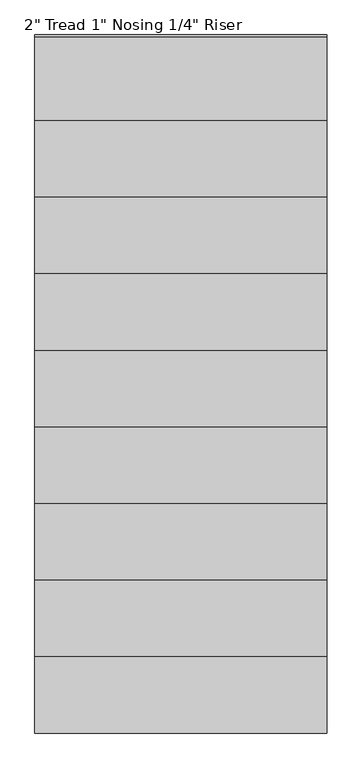
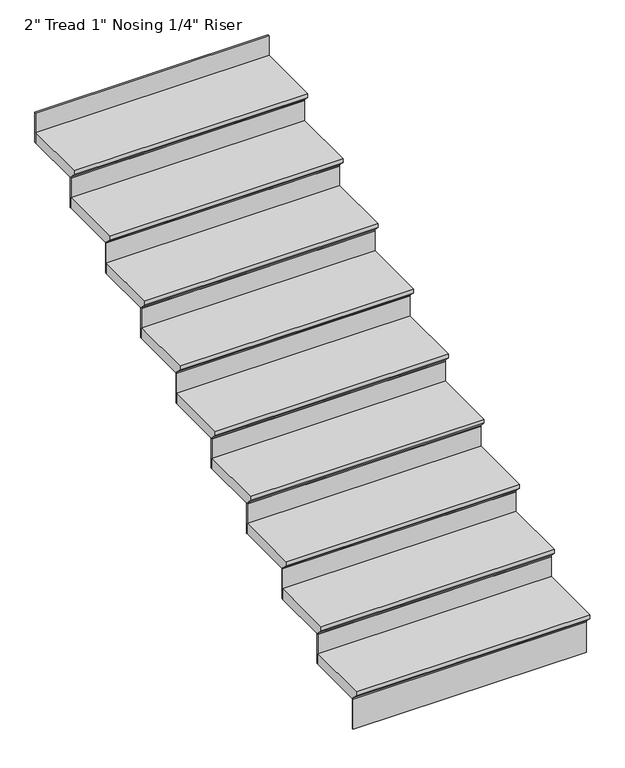
"""IFC4 building model written with IfcOpenShell, lengths in millimetres: stair flight geometry."""

from ifc_helpers import new_model, si_unit, frame, origin, place, context, project, spatial, polyline, outline, extrude, source, transform, mapped, element, save


def stair_flight_4fea8275(model_context):
    return source(origin(), model_context, "Body", "SweptSolid", [
        extrude(outline(polyline([(9995.9922903, 4800.6), (10300.7922903, 4800.6), (10300.7922903, 4749.8), (10021.3922903, 4749.8), (10021.3922903, 4756.15), (9995.9922903, 4781.55), (9995.9922903, 4800.6)])), frame((-17359.2847893, 0.0, 0.0), z_axis=(1.0, 0.0, 0.0), x_axis=(0.0, 1.0, 0.0)), (0.0, 0.0, 1.0), 1066.8),
        extrude(outline(polyline([(-16292.4847893, 10027.7422903), (-16292.4847893, 10021.3922903), (-17359.2847893, 10021.3922903), (-17359.2847893, 10027.7422903), (-16292.4847893, 10027.7422903)])), frame((0.0, 0.0, 4604.3272727), z_axis=(0.0, 0.0, 1.0), x_axis=(1.0, 0.0, 0.0)), (0.0, 0.0, 1.0), 145.4727273),
        extrude(outline(polyline([(-16292.4847893, 10307.1422903), (-16292.4847893, 10300.7922903), (-17359.2847893, 10300.7922903), (-17359.2847893, 10307.1422903), (-16292.4847893, 10307.1422903)])), frame((0.0, 0.0, 4749.8), z_axis=(0.0, 0.0, 1.0), x_axis=(1.0, 0.0, 0.0)), (0.0, 0.0, 1.0), 145.4727273),
        extrude(outline(polyline([(10275.3922903, 4946.0727273), (10580.1922903, 4946.0727273), (10580.1922903, 4895.2727273), (10300.7922903, 4895.2727273), (10300.7922903, 4901.6227273), (10275.3922903, 4927.0227273), (10275.3922903, 4946.0727273)])), frame((-17359.2847893, 0.0, 0.0), z_axis=(1.0, 0.0, 0.0), x_axis=(0.0, 1.0, 0.0)), (0.0, 0.0, 1.0), 1066.8),
        extrude(outline(polyline([(-16292.4847893, 10586.5422903), (-16292.4847893, 10580.1922903), (-17359.2847893, 10580.1922903), (-17359.2847893, 10586.5422903), (-16292.4847893, 10586.5422903)])), frame((0.0, 0.0, 4895.2727273), z_axis=(0.0, 0.0, 1.0), x_axis=(1.0, 0.0, 0.0)), (0.0, 0.0, 1.0), 145.4727273),
        extrude(outline(polyline([(10554.7922903, 5091.5454545), (10859.5922903, 5091.5454545), (10859.5922903, 5040.7454545), (10580.1922903, 5040.7454545), (10580.1922903, 5047.0954545), (10554.7922903, 5072.4954545), (10554.7922903, 5091.5454545)])), frame((-17359.2847893, 0.0, 0.0), z_axis=(1.0, 0.0, 0.0), x_axis=(0.0, 1.0, 0.0)), (0.0, 0.0, 1.0), 1066.8),
        extrude(outline(polyline([(-16292.4847893, 10865.9422903), (-16292.4847893, 10859.5922903), (-17359.2847893, 10859.5922903), (-17359.2847893, 10865.9422903), (-16292.4847893, 10865.9422903)])), frame((0.0, 0.0, 5040.7454545), z_axis=(0.0, 0.0, 1.0), x_axis=(1.0, 0.0, 0.0)), (0.0, 0.0, 1.0), 145.4727273),
        extrude(outline(polyline([(10834.1922903, 5237.0181818), (11138.9922903, 5237.0181818), (11138.9922903, 5186.2181818), (10859.5922903, 5186.2181818), (10859.5922903, 5192.5681818), (10834.1922903, 5217.9681818), (10834.1922903, 5237.0181818)])), frame((-17359.2847893, 0.0, 0.0), z_axis=(1.0, 0.0, 0.0), x_axis=(0.0, 1.0, 0.0)), (0.0, 0.0, 1.0), 1066.8),
        extrude(outline(polyline([(-16292.4847893, 11145.3422903), (-16292.4847893, 11138.9922903), (-17359.2847893, 11138.9922903), (-17359.2847893, 11145.3422903), (-16292.4847893, 11145.3422903)])), frame((0.0, 0.0, 5186.2181818), z_axis=(0.0, 0.0, 1.0), x_axis=(1.0, 0.0, 0.0)), (0.0, 0.0, 1.0), 145.4727273),
        extrude(outline(polyline([(11113.5922903, 5382.4909091), (11418.3922903, 5382.4909091), (11418.3922903, 5331.6909091), (11138.9922903, 5331.6909091), (11138.9922903, 5338.0409091), (11113.5922903, 5363.4409091), (11113.5922903, 5382.4909091)])), frame((-17359.2847893, 0.0, 0.0), z_axis=(1.0, 0.0, 0.0), x_axis=(0.0, 1.0, 0.0)), (0.0, 0.0, 1.0), 1066.8),
        extrude(outline(polyline([(-16292.4847893, 11424.7422903), (-16292.4847893, 11418.3922903), (-17359.2847893, 11418.3922903), (-17359.2847893, 11424.7422903), (-16292.4847893, 11424.7422903)])), frame((0.0, 0.0, 5331.6909091), z_axis=(0.0, 0.0, 1.0), x_axis=(1.0, 0.0, 0.0)), (0.0, 0.0, 1.0), 145.4727273),
        extrude(outline(polyline([(11392.9922903, 5527.9636364), (11697.7922903, 5527.9636364), (11697.7922903, 5477.1636364), (11418.3922903, 5477.1636364), (11418.3922903, 5483.5136364), (11392.9922903, 5508.9136364), (11392.9922903, 5527.9636364)])), frame((-17359.2847893, 0.0, 0.0), z_axis=(1.0, 0.0, 0.0), x_axis=(0.0, 1.0, 0.0)), (0.0, 0.0, 1.0), 1066.8),
        extrude(outline(polyline([(-16292.4847893, 11704.1422903), (-16292.4847893, 11697.7922903), (-17359.2847893, 11697.7922903), (-17359.2847893, 11704.1422903), (-16292.4847893, 11704.1422903)])), frame((0.0, 0.0, 5477.1636364), z_axis=(0.0, 0.0, 1.0), x_axis=(1.0, 0.0, 0.0)), (0.0, 0.0, 1.0), 145.4727273),
        extrude(outline(polyline([(11672.3922903, 5673.4363636), (11977.1922903, 5673.4363636), (11977.1922903, 5622.6363636), (11697.7922903, 5622.6363636), (11697.7922903, 5628.9863636), (11672.3922903, 5654.3863636), (11672.3922903, 5673.4363636)])), frame((-17359.2847893, 0.0, 0.0), z_axis=(1.0, 0.0, 0.0), x_axis=(0.0, 1.0, 0.0)), (0.0, 0.0, 1.0), 1066.8),
        extrude(outline(polyline([(-16292.4847893, 11983.5422903), (-16292.4847893, 11977.1922903), (-17359.2847893, 11977.1922903), (-17359.2847893, 11983.5422903), (-16292.4847893, 11983.5422903)])), frame((0.0, 0.0, 5622.6363636), z_axis=(0.0, 0.0, 1.0), x_axis=(1.0, 0.0, 0.0)), (0.0, 0.0, 1.0), 145.4727273),
        extrude(outline(polyline([(11951.7922903, 5818.9090909), (12256.5922903, 5818.9090909), (12256.5922903, 5768.1090909), (11977.1922903, 5768.1090909), (11977.1922903, 5774.4590909), (11951.7922903, 5799.8590909), (11951.7922903, 5818.9090909)])), frame((-17359.2847893, 0.0, 0.0), z_axis=(1.0, 0.0, 0.0), x_axis=(0.0, 1.0, 0.0)), (0.0, 0.0, 1.0), 1066.8),
        extrude(outline(polyline([(-16292.4847893, 12262.9422903), (-16292.4847893, 12256.5922903), (-17359.2847893, 12256.5922903), (-17359.2847893, 12262.9422903), (-16292.4847893, 12262.9422903)])), frame((0.0, 0.0, 5768.1090909), z_axis=(0.0, 0.0, 1.0), x_axis=(1.0, 0.0, 0.0)), (0.0, 0.0, 1.0), 145.4727273),
        extrude(outline(polyline([(-16292.4847893, 12542.3422903), (-16292.4847893, 12535.9922903), (-17359.2847893, 12535.9922903), (-17359.2847893, 12542.3422903), (-16292.4847893, 12542.3422903)])), frame((0.0, 0.0, 5913.5818182), z_axis=(0.0, 0.0, 1.0), x_axis=(1.0, 0.0, 0.0)), (0.0, 0.0, 1.0), 145.4727273),
        extrude(outline(polyline([(12231.1922903, 5964.3818182), (12535.9922903, 5964.3818182), (12535.9922903, 5913.5818182), (12256.5922903, 5913.5818182), (12256.5922903, 5919.9318182), (12231.1922903, 5945.3318182), (12231.1922903, 5964.3818182)])), frame((-17359.2847893, 0.0, 0.0), z_axis=(1.0, 0.0, 0.0), x_axis=(0.0, 1.0, 0.0)), (0.0, 0.0, 1.0), 1066.8),
    ])


if __name__ == "__main__":
    model = new_model("IFC4")
    model_context = context("Model", 3, world=origin())
    ifc_project = project(units=[si_unit("LENGTHUNIT", "METRE", prefix="MILLI")], contexts=[model_context])
    site = spatial("IfcSite", under=ifc_project)
    building = spatial("IfcBuilding", under=site)
    placement = place(None, origin())
    stair_flight_shape = stair_flight_4fea8275(model_context)
    element("IfcStairFlight", 1, ObjectType="2\" Tread 1\" Nosing 1/4\" Riser", at=placement, inside=building, context=model_context, shape_type="MappedRepresentation", body=[
        mapped(stair_flight_shape, transform((0.0, 0.0, 0.0), x_axis=(1.0, 0.0, 0.0), y_axis=(0.0, 1.0, 0.0), z_axis=(0.0, 0.0, 1.0))),
    ])
    save(model, "model.ifc")
